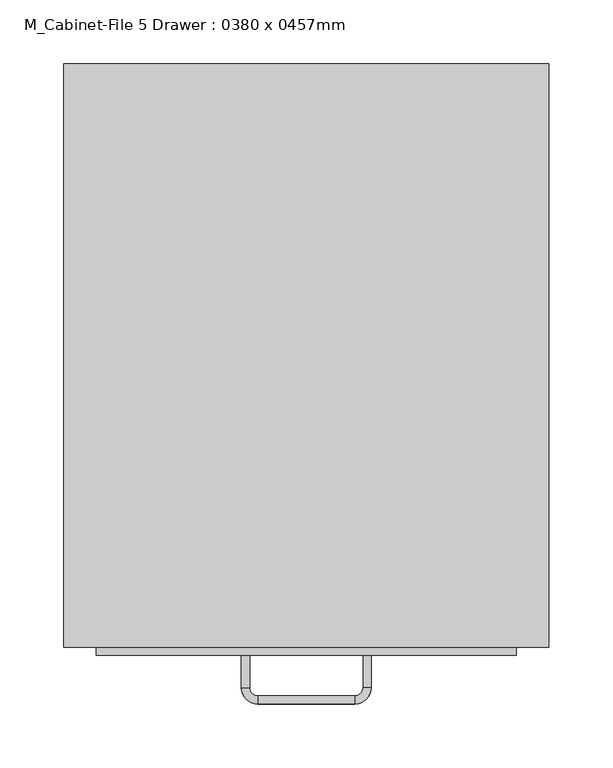
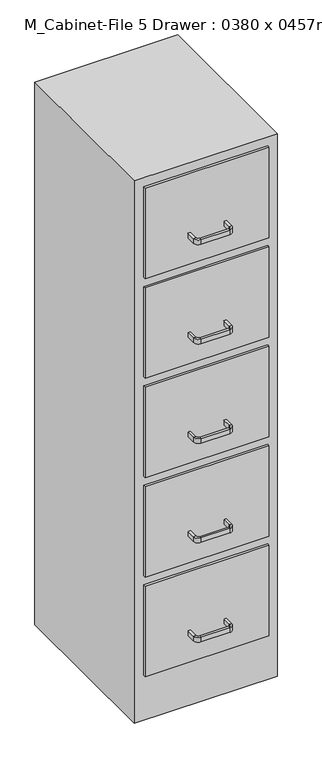
"""IFC4 building model written with IfcOpenShell, lengths in millimetres: furniture geometry, M_Cabinet-File 5 Drawer : 0380 x 0457mm."""

from ifc_helpers import new_model, si_unit, frame, origin, origin_with_axes, place, context, project, spatial, polyline, circle_curve, outline, extrude, source, transform, mapped, element, save
from ifc_brep_helpers import plane_surface, cylinder_surface, revolved_surface, advanced_brep


def m_cabinet_file_5_drawer_0380_x_0457mm_21dee09a(model_context):
    return source(origin(), model_context, "Body", "SolidModel", [
        extrude(outline(polyline([(36.703553, -376.9843001), (-292.496447, -376.9843001), (-292.496447, -370.6343001), (36.703553, -370.6343001), (36.703553, -376.9843001)])), frame((0.0, 0.0, 1244.6), z_axis=(0.0, 0.0, 1.0), x_axis=(1.0, 0.0, 0.0)), (0.0, 0.0, 1.0), 255.0),
        extrude(outline(polyline([(36.703553, -376.9843001), (-292.496447, -376.9843001), (-292.496447, -370.6343001), (36.703553, -370.6343001), (36.703553, -376.9843001)])), frame((0.0, 0.0, 965.2), z_axis=(0.0, 0.0, 1.0), x_axis=(1.0, 0.0, 0.0)), (0.0, 0.0, 1.0), 254.0),
        extrude(outline(polyline([(36.703553, -376.9843001), (-292.496447, -376.9843001), (-292.496447, -370.6343001), (36.703553, -370.6343001), (36.703553, -376.9843001)])), frame((0.0, 0.0, 685.8), z_axis=(0.0, 0.0, 1.0), x_axis=(1.0, 0.0, 0.0)), (0.0, 0.0, 1.0), 254.0),
        extrude(outline(polyline([(36.703553, -376.9843001), (-292.496447, -376.9843001), (-292.496447, -370.6343001), (36.703553, -370.6343001), (36.703553, -376.9843001)])), frame((0.0, 0.0, 406.4), z_axis=(0.0, 0.0, 1.0), x_axis=(1.0, 0.0, 0.0)), (0.0, 0.0, 1.0), 254.0),
        extrude(outline(polyline([(36.703553, -376.9843001), (-292.496447, -376.9843001), (-292.496447, -370.6343001), (36.703553, -370.6343001), (36.703553, -376.9843001)])), frame((0.0, 0.0, 127.0), z_axis=(0.0, 0.0, 1.0), x_axis=(1.0, 0.0, 0.0)), (0.0, 0.0, 1.0), 254.0),
        extrude(outline(polyline([(62.103553, 86.3656999), (62.103553, -370.6343001), (-317.896447, -370.6343001), (-317.896447, 86.3656999), (62.103553, 86.3656999)])), origin_with_axes(), (0.0, 0.0, 1.0), 1525.0),
        advanced_brep(
        [(-172.346447, -376.9843001, 203.2), (-178.696447, -376.9843001, 203.2), (-178.696447, -376.9843001, 215.9), (-172.346447, -376.9843001, 215.9), (-172.346447, -402.3843001, 203.2), (-178.696447, -402.3843001, 203.2), (-178.696447, -402.3843001, 215.9), (-172.346447, -402.3843001, 215.9), (-165.996447, -415.0843001, 203.2), (-165.996447, -408.7343001, 203.2), (-165.996447, -415.0843001, 215.9), (-165.996447, -408.7343001, 215.9), (-89.796447, -408.7343001, 203.2), (-89.796447, -415.0843001, 203.2), (-89.796447, -415.0843001, 215.9), (-89.796447, -408.7343001, 215.9), (-77.096447, -402.3843001, 203.2), (-83.446447, -402.3843001, 203.2), (-77.096447, -402.3843001, 215.9), (-83.446447, -402.3843001, 215.9), (-83.446447, -376.9843001, 203.2), (-83.446447, -376.9843001, 215.9), (-77.096447, -376.9843001, 215.9), (-77.096447, -376.9843001, 203.2)],
        [
            (0, 1),
            (1, 2),
            (2, 3),
            (3, 0),
            (0, 4),
            (4, 5),
            (5, 1),
            (5, 6),
            (6, 2),
            (6, 7),
            (7, 3),
            (7, 4),
            (8, 5, circle_curve(frame((-165.996447, -402.3843001, 203.2), z_axis=(0.0, 0.0, -1.0), x_axis=(-1.0, 0.0, 0.0)), 12.7)),
            (4, 9, circle_curve(frame((-165.996447, -402.3843001, 203.2), z_axis=(0.0, 0.0, 1.0), x_axis=(-1.0, 0.0, 0.0)), 6.35)),
            (9, 8),
            (10, 6, circle_curve(frame((-165.996447, -402.3843001, 215.9), z_axis=(0.0, 0.0, -1.0), x_axis=(-1.0, 0.0, 0.0)), 12.7)),
            (8, 10),
            (11, 7, circle_curve(frame((-165.996447, -402.3843001, 215.9), z_axis=(0.0, 0.0, -1.0), x_axis=(-1.0, 0.0, 0.0)), 6.35)),
            (10, 11),
            (11, 9),
            (9, 12),
            (12, 13),
            (13, 8),
            (13, 14),
            (14, 10),
            (14, 15),
            (15, 11),
            (15, 12),
            (16, 13, circle_curve(frame((-89.796447, -402.3843001, 203.2), z_axis=(0.0, 0.0, -1.0), x_axis=(0.0, -1.0, 0.0)), 12.7)),
            (12, 17, circle_curve(frame((-89.796447, -402.3843001, 203.2), z_axis=(0.0, 0.0, 1.0), x_axis=(0.0, -1.0, 0.0)), 6.35)),
            (17, 16),
            (18, 14, circle_curve(frame((-89.796447, -402.3843001, 215.9), z_axis=(0.0, 0.0, -1.0), x_axis=(0.0, -1.0, 0.0)), 12.7)),
            (16, 18),
            (19, 15, circle_curve(frame((-89.796447, -402.3843001, 215.9), z_axis=(0.0, 0.0, -1.0), x_axis=(0.0, -1.0, 0.0)), 6.35)),
            (18, 19),
            (19, 17),
            (20, 21),
            (21, 22),
            (22, 23),
            (23, 20),
            (17, 20),
            (23, 16),
            (22, 18),
            (21, 19),
        ],
        [
            plane_surface(frame((-1512.211566, -376.9843001, 0.0), z_axis=(0.0, 1.0, 0.0), x_axis=(0.0, 0.0, -1.0))),
            plane_surface(frame((-172.346447, -376.9843001, 203.2), z_axis=(0.0, 0.0, -1.0), x_axis=(0.0, -1.0, 0.0))),
            plane_surface(frame((-178.696447, -376.9843001, 203.2), z_axis=(-1.0, 0.0, 0.0), x_axis=(0.0, -1.0, 0.0))),
            plane_surface(frame((-178.696447, -376.9843001, 215.9), z_axis=(0.0, 0.0, 1.0), x_axis=(0.0, -1.0, 0.0))),
            plane_surface(frame((-172.346447, -376.9843001, 215.9), z_axis=(1.0, 0.0, 0.0), x_axis=(0.0, -1.0, 0.0))),
            plane_surface(frame((-165.996447, -402.3843001, 203.2), z_axis=(0.0, 0.0, -1.0), x_axis=(-1.0, 0.0, 0.0))),
            cylinder_surface(frame((-165.996447, -402.3843001, 0.0), z_axis=(0.0, 0.0, 1.0), x_axis=(-1.0, 0.0, 0.0)), 12.7),
            plane_surface(frame((-165.996447, -402.3843001, 215.9), z_axis=(0.0, 0.0, 1.0), x_axis=(-1.0, 0.0, 0.0))),
            revolved_surface(polyline([(-172.34644699999998, -402.3843001, 215.9), (-172.34644699999998, -402.3843001, 203.2)]), (-165.996447, -402.3843001, 0.0), (0.0, 0.0, 1.0)),
            plane_surface(frame((-165.996447, -408.7343001, 203.2), z_axis=(0.0, 0.0, -1.0), x_axis=(1.0, 0.0, 0.0))),
            plane_surface(frame((-165.996447, -415.0843001, 203.2), z_axis=(0.0, -1.0, 0.0), x_axis=(1.0, 0.0, 0.0))),
            plane_surface(frame((-165.996447, -415.0843001, 215.9), z_axis=(0.0, 0.0, 1.0), x_axis=(1.0, 0.0, 0.0))),
            plane_surface(frame((-165.996447, -408.7343001, 215.9), z_axis=(0.0, 1.0, 0.0), x_axis=(1.0, 0.0, 0.0))),
            plane_surface(frame((-89.796447, -402.3843001, 203.2), z_axis=(0.0, 0.0, -1.0), x_axis=(0.0, -1.0, 0.0))),
            cylinder_surface(frame((-89.796447, -402.3843001, 0.0), z_axis=(0.0, 0.0, 1.0), x_axis=(0.0, -1.0, 0.0)), 12.7),
            plane_surface(frame((-89.796447, -402.3843001, 215.9), z_axis=(0.0, 0.0, 1.0), x_axis=(0.0, -1.0, 0.0))),
            revolved_surface(polyline([(-89.796447, -408.73430010000004, 215.9), (-89.796447, -408.73430010000004, 203.2)]), (-89.796447, -402.3843001, 0.0), (0.0, 0.0, 1.0)),
            plane_surface(frame((-1410.611566, -376.9843001, 0.0), z_axis=(0.0, 1.0, 0.0), x_axis=(0.0, 0.0, 1.0))),
            plane_surface(frame((-83.446447, -402.3843001, 203.2), z_axis=(0.0, 0.0, -1.0), x_axis=(0.0, 1.0, 0.0))),
            plane_surface(frame((-77.096447, -402.3843001, 203.2), z_axis=(1.0, 0.0, 0.0), x_axis=(0.0, 1.0, 0.0))),
            plane_surface(frame((-77.096447, -402.3843001, 215.9), z_axis=(0.0, 0.0, 1.0), x_axis=(0.0, 1.0, 0.0))),
            plane_surface(frame((-83.446447, -402.3843001, 215.9), z_axis=(-1.0, 0.0, 0.0), x_axis=(0.0, 1.0, 0.0))),
        ],
        [
            (0, [[1, 2, 3, 4]]),
            (1, [[-1, 5, 6, 7]]),
            (2, [[-2, -7, 8, 9]]),
            (3, [[-3, -9, 10, 11]]),
            (4, [[-4, -11, 12, -5]]),
            (5, [[13, -6, 14, 15]]),
            (6, [[16, -8, -13, 17]]),
            (7, [[18, -10, -16, 19]]),
            (8, [[-14, -12, -18, 20]]),
            (9, [[-15, 21, 22, 23]]),
            (10, [[-17, -23, 24, 25]]),
            (11, [[-19, -25, 26, 27]]),
            (12, [[-20, -27, 28, -21]]),
            (13, [[29, -22, 30, 31]]),
            (14, [[32, -24, -29, 33]]),
            (15, [[34, -26, -32, 35]]),
            (16, [[-30, -28, -34, 36]]),
            (17, [[37, 38, 39, 40]]),
            (18, [[-31, 41, -40, 42]]),
            (19, [[-33, -42, -39, 43]]),
            (20, [[-35, -43, -38, 44]]),
            (21, [[-36, -44, -37, -41]]),
        ],
    ),
        advanced_brep(
        [(-172.346447, -376.9843001, 482.6), (-178.696447, -376.9843001, 482.6), (-178.696447, -376.9843001, 495.3), (-172.346447, -376.9843001, 495.3), (-172.346447, -402.3843001, 482.6), (-178.696447, -402.3843001, 482.6), (-178.696447, -402.3843001, 495.3), (-172.346447, -402.3843001, 495.3), (-165.996447, -415.0843001, 482.6), (-165.996447, -408.7343001, 482.6), (-165.996447, -415.0843001, 495.3), (-165.996447, -408.7343001, 495.3), (-89.796447, -408.7343001, 482.6), (-89.796447, -415.0843001, 482.6), (-89.796447, -415.0843001, 495.3), (-89.796447, -408.7343001, 495.3), (-77.096447, -402.3843001, 482.6), (-83.446447, -402.3843001, 482.6), (-77.096447, -402.3843001, 495.3), (-83.446447, -402.3843001, 495.3), (-83.446447, -376.9843001, 482.6), (-83.446447, -376.9843001, 495.3), (-77.096447, -376.9843001, 495.3), (-77.096447, -376.9843001, 482.6)],
        [
            (0, 1),
            (1, 2),
            (2, 3),
            (3, 0),
            (0, 4),
            (4, 5),
            (5, 1),
            (5, 6),
            (6, 2),
            (6, 7),
            (7, 3),
            (7, 4),
            (8, 5, circle_curve(frame((-165.996447, -402.3843001, 482.6), z_axis=(0.0, 0.0, -1.0), x_axis=(-1.0, 0.0, 0.0)), 12.7)),
            (4, 9, circle_curve(frame((-165.996447, -402.3843001, 482.6), z_axis=(0.0, 0.0, 1.0), x_axis=(-1.0, 0.0, 0.0)), 6.35)),
            (9, 8),
            (10, 6, circle_curve(frame((-165.996447, -402.3843001, 495.3), z_axis=(0.0, 0.0, -1.0), x_axis=(-1.0, 0.0, 0.0)), 12.7)),
            (8, 10),
            (11, 7, circle_curve(frame((-165.996447, -402.3843001, 495.3), z_axis=(0.0, 0.0, -1.0), x_axis=(-1.0, 0.0, 0.0)), 6.35)),
            (10, 11),
            (11, 9),
            (9, 12),
            (12, 13),
            (13, 8),
            (13, 14),
            (14, 10),
            (14, 15),
            (15, 11),
            (15, 12),
            (16, 13, circle_curve(frame((-89.796447, -402.3843001, 482.6), z_axis=(0.0, 0.0, -1.0), x_axis=(0.0, -1.0, 0.0)), 12.7)),
            (12, 17, circle_curve(frame((-89.796447, -402.3843001, 482.6), z_axis=(0.0, 0.0, 1.0), x_axis=(0.0, -1.0, 0.0)), 6.35)),
            (17, 16),
            (18, 14, circle_curve(frame((-89.796447, -402.3843001, 495.3), z_axis=(0.0, 0.0, -1.0), x_axis=(0.0, -1.0, 0.0)), 12.7)),
            (16, 18),
            (19, 15, circle_curve(frame((-89.796447, -402.3843001, 495.3), z_axis=(0.0, 0.0, -1.0), x_axis=(0.0, -1.0, 0.0)), 6.35)),
            (18, 19),
            (19, 17),
            (20, 21),
            (21, 22),
            (22, 23),
            (23, 20),
            (17, 20),
            (23, 16),
            (22, 18),
            (21, 19),
        ],
        [
            plane_surface(frame((-1512.211566, -376.9843001, 0.0), z_axis=(0.0, 1.0, 0.0), x_axis=(0.0, 0.0, -1.0))),
            plane_surface(frame((-172.346447, -376.9843001, 482.6), z_axis=(0.0, 0.0, -1.0), x_axis=(0.0, -1.0, 0.0))),
            plane_surface(frame((-178.696447, -376.9843001, 482.6), z_axis=(-1.0, 0.0, 0.0), x_axis=(0.0, -1.0, 0.0))),
            plane_surface(frame((-178.696447, -376.9843001, 495.3), z_axis=(0.0, 0.0, 1.0), x_axis=(0.0, -1.0, 0.0))),
            plane_surface(frame((-172.346447, -376.9843001, 495.3), z_axis=(1.0, 0.0, 0.0), x_axis=(0.0, -1.0, 0.0))),
            plane_surface(frame((-165.996447, -402.3843001, 482.6), z_axis=(0.0, 0.0, -1.0), x_axis=(-1.0, 0.0, 0.0))),
            cylinder_surface(frame((-165.996447, -402.3843001, 0.0), z_axis=(0.0, 0.0, 1.0), x_axis=(-1.0, 0.0, 0.0)), 12.7),
            plane_surface(frame((-165.996447, -402.3843001, 495.3), z_axis=(0.0, 0.0, 1.0), x_axis=(-1.0, 0.0, 0.0))),
            revolved_surface(polyline([(-172.34644699999998, -402.3843001, 495.3), (-172.34644699999998, -402.3843001, 482.6)]), (-165.996447, -402.3843001, 0.0), (0.0, 0.0, 1.0)),
            plane_surface(frame((-165.996447, -408.7343001, 482.6), z_axis=(0.0, 0.0, -1.0), x_axis=(1.0, 0.0, 0.0))),
            plane_surface(frame((-165.996447, -415.0843001, 482.6), z_axis=(0.0, -1.0, 0.0), x_axis=(1.0, 0.0, 0.0))),
            plane_surface(frame((-165.996447, -415.0843001, 495.3), z_axis=(0.0, 0.0, 1.0), x_axis=(1.0, 0.0, 0.0))),
            plane_surface(frame((-165.996447, -408.7343001, 495.3), z_axis=(0.0, 1.0, 0.0), x_axis=(1.0, 0.0, 0.0))),
            plane_surface(frame((-89.796447, -402.3843001, 482.6), z_axis=(0.0, 0.0, -1.0), x_axis=(0.0, -1.0, 0.0))),
            cylinder_surface(frame((-89.796447, -402.3843001, 0.0), z_axis=(0.0, 0.0, 1.0), x_axis=(0.0, -1.0, 0.0)), 12.7),
            plane_surface(frame((-89.796447, -402.3843001, 495.3), z_axis=(0.0, 0.0, 1.0), x_axis=(0.0, -1.0, 0.0))),
            revolved_surface(polyline([(-89.796447, -408.73430010000004, 495.3), (-89.796447, -408.73430010000004, 482.6)]), (-89.796447, -402.3843001, 0.0), (0.0, 0.0, 1.0)),
            plane_surface(frame((-1410.611566, -376.9843001, 0.0), z_axis=(0.0, 1.0, 0.0), x_axis=(0.0, 0.0, 1.0))),
            plane_surface(frame((-83.446447, -402.3843001, 482.6), z_axis=(0.0, 0.0, -1.0), x_axis=(0.0, 1.0, 0.0))),
            plane_surface(frame((-77.096447, -402.3843001, 482.6), z_axis=(1.0, 0.0, 0.0), x_axis=(0.0, 1.0, 0.0))),
            plane_surface(frame((-77.096447, -402.3843001, 495.3), z_axis=(0.0, 0.0, 1.0), x_axis=(0.0, 1.0, 0.0))),
            plane_surface(frame((-83.446447, -402.3843001, 495.3), z_axis=(-1.0, 0.0, 0.0), x_axis=(0.0, 1.0, 0.0))),
        ],
        [
            (0, [[1, 2, 3, 4]]),
            (1, [[-1, 5, 6, 7]]),
            (2, [[-2, -7, 8, 9]]),
            (3, [[-3, -9, 10, 11]]),
            (4, [[-4, -11, 12, -5]]),
            (5, [[13, -6, 14, 15]]),
            (6, [[16, -8, -13, 17]]),
            (7, [[18, -10, -16, 19]]),
            (8, [[-14, -12, -18, 20]]),
            (9, [[-15, 21, 22, 23]]),
            (10, [[-17, -23, 24, 25]]),
            (11, [[-19, -25, 26, 27]]),
            (12, [[-20, -27, 28, -21]]),
            (13, [[29, -22, 30, 31]]),
            (14, [[32, -24, -29, 33]]),
            (15, [[34, -26, -32, 35]]),
            (16, [[-30, -28, -34, 36]]),
            (17, [[37, 38, 39, 40]]),
            (18, [[-31, 41, -40, 42]]),
            (19, [[-33, -42, -39, 43]]),
            (20, [[-35, -43, -38, 44]]),
            (21, [[-36, -44, -37, -41]]),
        ],
    ),
        advanced_brep(
        [(-172.346447, -376.9843001, 762.0), (-178.696447, -376.9843001, 762.0), (-178.696447, -376.9843001, 774.7), (-172.346447, -376.9843001, 774.7), (-172.346447, -402.3843001, 762.0), (-178.696447, -402.3843001, 762.0), (-178.696447, -402.3843001, 774.7), (-172.346447, -402.3843001, 774.7), (-165.996447, -415.0843001, 762.0), (-165.996447, -408.7343001, 762.0), (-165.996447, -415.0843001, 774.7), (-165.996447, -408.7343001, 774.7), (-89.796447, -408.7343001, 762.0), (-89.796447, -415.0843001, 762.0), (-89.796447, -415.0843001, 774.7), (-89.796447, -408.7343001, 774.7), (-77.096447, -402.3843001, 762.0), (-83.446447, -402.3843001, 762.0), (-77.096447, -402.3843001, 774.7), (-83.446447, -402.3843001, 774.7), (-83.446447, -376.9843001, 762.0), (-83.446447, -376.9843001, 774.7), (-77.096447, -376.9843001, 774.7), (-77.096447, -376.9843001, 762.0)],
        [
            (0, 1),
            (1, 2),
            (2, 3),
            (3, 0),
            (0, 4),
            (4, 5),
            (5, 1),
            (5, 6),
            (6, 2),
            (6, 7),
            (7, 3),
            (7, 4),
            (8, 5, circle_curve(frame((-165.996447, -402.3843001, 762.0), z_axis=(0.0, 0.0, -1.0), x_axis=(-1.0, 0.0, 0.0)), 12.7)),
            (4, 9, circle_curve(frame((-165.996447, -402.3843001, 762.0), z_axis=(0.0, 0.0, 1.0), x_axis=(-1.0, 0.0, 0.0)), 6.35)),
            (9, 8),
            (10, 6, circle_curve(frame((-165.996447, -402.3843001, 774.7), z_axis=(0.0, 0.0, -1.0), x_axis=(-1.0, 0.0, 0.0)), 12.7)),
            (8, 10),
            (11, 7, circle_curve(frame((-165.996447, -402.3843001, 774.7), z_axis=(0.0, 0.0, -1.0), x_axis=(-1.0, 0.0, 0.0)), 6.35)),
            (10, 11),
            (11, 9),
            (9, 12),
            (12, 13),
            (13, 8),
            (13, 14),
            (14, 10),
            (14, 15),
            (15, 11),
            (15, 12),
            (16, 13, circle_curve(frame((-89.796447, -402.3843001, 762.0), z_axis=(0.0, 0.0, -1.0), x_axis=(0.0, -1.0, 0.0)), 12.7)),
            (12, 17, circle_curve(frame((-89.796447, -402.3843001, 762.0), z_axis=(0.0, 0.0, 1.0), x_axis=(0.0, -1.0, 0.0)), 6.35)),
            (17, 16),
            (18, 14, circle_curve(frame((-89.796447, -402.3843001, 774.7), z_axis=(0.0, 0.0, -1.0), x_axis=(0.0, -1.0, 0.0)), 12.7)),
            (16, 18),
            (19, 15, circle_curve(frame((-89.796447, -402.3843001, 774.7), z_axis=(0.0, 0.0, -1.0), x_axis=(0.0, -1.0, 0.0)), 6.35)),
            (18, 19),
            (19, 17),
            (20, 21),
            (21, 22),
            (22, 23),
            (23, 20),
            (17, 20),
            (23, 16),
            (22, 18),
            (21, 19),
        ],
        [
            plane_surface(frame((-1512.211566, -376.9843001, 0.0), z_axis=(0.0, 1.0, 0.0), x_axis=(0.0, 0.0, -1.0))),
            plane_surface(frame((-172.346447, -376.9843001, 762.0), z_axis=(0.0, 0.0, -1.0), x_axis=(0.0, -1.0, 0.0))),
            plane_surface(frame((-178.696447, -376.9843001, 762.0), z_axis=(-1.0, 0.0, 0.0), x_axis=(0.0, -1.0, 0.0))),
            plane_surface(frame((-178.696447, -376.9843001, 774.7), z_axis=(0.0, 0.0, 1.0), x_axis=(0.0, -1.0, 0.0))),
            plane_surface(frame((-172.346447, -376.9843001, 774.7), z_axis=(1.0, 0.0, 0.0), x_axis=(0.0, -1.0, 0.0))),
            plane_surface(frame((-165.996447, -402.3843001, 762.0), z_axis=(0.0, 0.0, -1.0), x_axis=(-1.0, 0.0, 0.0))),
            cylinder_surface(frame((-165.996447, -402.3843001, 0.0), z_axis=(0.0, 0.0, 1.0), x_axis=(-1.0, 0.0, 0.0)), 12.7),
            plane_surface(frame((-165.996447, -402.3843001, 774.7), z_axis=(0.0, 0.0, 1.0), x_axis=(-1.0, 0.0, 0.0))),
            revolved_surface(polyline([(-172.34644699999998, -402.3843001, 774.7), (-172.34644699999998, -402.3843001, 762.0)]), (-165.996447, -402.3843001, 0.0), (0.0, 0.0, 1.0)),
            plane_surface(frame((-165.996447, -408.7343001, 762.0), z_axis=(0.0, 0.0, -1.0), x_axis=(1.0, 0.0, 0.0))),
            plane_surface(frame((-165.996447, -415.0843001, 762.0), z_axis=(0.0, -1.0, 0.0), x_axis=(1.0, 0.0, 0.0))),
            plane_surface(frame((-165.996447, -415.0843001, 774.7), z_axis=(0.0, 0.0, 1.0), x_axis=(1.0, 0.0, 0.0))),
            plane_surface(frame((-165.996447, -408.7343001, 774.7), z_axis=(0.0, 1.0, 0.0), x_axis=(1.0, 0.0, 0.0))),
            plane_surface(frame((-89.796447, -402.3843001, 762.0), z_axis=(0.0, 0.0, -1.0), x_axis=(0.0, -1.0, 0.0))),
            cylinder_surface(frame((-89.796447, -402.3843001, 0.0), z_axis=(0.0, 0.0, 1.0), x_axis=(0.0, -1.0, 0.0)), 12.7),
            plane_surface(frame((-89.796447, -402.3843001, 774.7), z_axis=(0.0, 0.0, 1.0), x_axis=(0.0, -1.0, 0.0))),
            revolved_surface(polyline([(-89.796447, -408.73430010000004, 774.7), (-89.796447, -408.73430010000004, 762.0)]), (-89.796447, -402.3843001, 0.0), (0.0, 0.0, 1.0)),
            plane_surface(frame((-1410.611566, -376.9843001, 0.0), z_axis=(0.0, 1.0, 0.0), x_axis=(0.0, 0.0, 1.0))),
            plane_surface(frame((-83.446447, -402.3843001, 762.0), z_axis=(0.0, 0.0, -1.0), x_axis=(0.0, 1.0, 0.0))),
            plane_surface(frame((-77.096447, -402.3843001, 762.0), z_axis=(1.0, 0.0, 0.0), x_axis=(0.0, 1.0, 0.0))),
            plane_surface(frame((-77.096447, -402.3843001, 774.7), z_axis=(0.0, 0.0, 1.0), x_axis=(0.0, 1.0, 0.0))),
            plane_surface(frame((-83.446447, -402.3843001, 774.7), z_axis=(-1.0, 0.0, 0.0), x_axis=(0.0, 1.0, 0.0))),
        ],
        [
            (0, [[1, 2, 3, 4]]),
            (1, [[-1, 5, 6, 7]]),
            (2, [[-2, -7, 8, 9]]),
            (3, [[-3, -9, 10, 11]]),
            (4, [[-4, -11, 12, -5]]),
            (5, [[13, -6, 14, 15]]),
            (6, [[16, -8, -13, 17]]),
            (7, [[18, -10, -16, 19]]),
            (8, [[-14, -12, -18, 20]]),
            (9, [[-15, 21, 22, 23]]),
            (10, [[-17, -23, 24, 25]]),
            (11, [[-19, -25, 26, 27]]),
            (12, [[-20, -27, 28, -21]]),
            (13, [[29, -22, 30, 31]]),
            (14, [[32, -24, -29, 33]]),
            (15, [[34, -26, -32, 35]]),
            (16, [[-30, -28, -34, 36]]),
            (17, [[37, 38, 39, 40]]),
            (18, [[-31, 41, -40, 42]]),
            (19, [[-33, -42, -39, 43]]),
            (20, [[-35, -43, -38, 44]]),
            (21, [[-36, -44, -37, -41]]),
        ],
    ),
        advanced_brep(
        [(-172.346447, -376.9843001, 1041.4), (-178.696447, -376.9843001, 1041.4), (-178.696447, -376.9843001, 1054.1), (-172.346447, -376.9843001, 1054.1), (-172.346447, -402.3843001, 1041.4), (-178.696447, -402.3843001, 1041.4), (-178.696447, -402.3843001, 1054.1), (-172.346447, -402.3843001, 1054.1), (-165.996447, -415.0843001, 1041.4), (-165.996447, -408.7343001, 1041.4), (-165.996447, -415.0843001, 1054.1), (-165.996447, -408.7343001, 1054.1), (-89.796447, -408.7343001, 1041.4), (-89.796447, -415.0843001, 1041.4), (-89.796447, -415.0843001, 1054.1), (-89.796447, -408.7343001, 1054.1), (-77.096447, -402.3843001, 1041.4), (-83.446447, -402.3843001, 1041.4), (-77.096447, -402.3843001, 1054.1), (-83.446447, -402.3843001, 1054.1), (-83.446447, -376.9843001, 1041.4), (-83.446447, -376.9843001, 1054.1), (-77.096447, -376.9843001, 1054.1), (-77.096447, -376.9843001, 1041.4)],
        [
            (0, 1),
            (1, 2),
            (2, 3),
            (3, 0),
            (0, 4),
            (4, 5),
            (5, 1),
            (5, 6),
            (6, 2),
            (6, 7),
            (7, 3),
            (7, 4),
            (8, 5, circle_curve(frame((-165.996447, -402.3843001, 1041.4), z_axis=(0.0, 0.0, -1.0), x_axis=(-1.0, 0.0, 0.0)), 12.7)),
            (4, 9, circle_curve(frame((-165.996447, -402.3843001, 1041.4), z_axis=(0.0, 0.0, 1.0), x_axis=(-1.0, 0.0, 0.0)), 6.35)),
            (9, 8),
            (10, 6, circle_curve(frame((-165.996447, -402.3843001, 1054.1), z_axis=(0.0, 0.0, -1.0), x_axis=(-1.0, 0.0, 0.0)), 12.7)),
            (8, 10),
            (11, 7, circle_curve(frame((-165.996447, -402.3843001, 1054.1), z_axis=(0.0, 0.0, -1.0), x_axis=(-1.0, 0.0, 0.0)), 6.35)),
            (10, 11),
            (11, 9),
            (9, 12),
            (12, 13),
            (13, 8),
            (13, 14),
            (14, 10),
            (14, 15),
            (15, 11),
            (15, 12),
            (16, 13, circle_curve(frame((-89.796447, -402.3843001, 1041.4), z_axis=(0.0, 0.0, -1.0), x_axis=(0.0, -1.0, 0.0)), 12.7)),
            (12, 17, circle_curve(frame((-89.796447, -402.3843001, 1041.4), z_axis=(0.0, 0.0, 1.0), x_axis=(0.0, -1.0, 0.0)), 6.35)),
            (17, 16),
            (18, 14, circle_curve(frame((-89.796447, -402.3843001, 1054.1), z_axis=(0.0, 0.0, -1.0), x_axis=(0.0, -1.0, 0.0)), 12.7)),
            (16, 18),
            (19, 15, circle_curve(frame((-89.796447, -402.3843001, 1054.1), z_axis=(0.0, 0.0, -1.0), x_axis=(0.0, -1.0, 0.0)), 6.35)),
            (18, 19),
            (19, 17),
            (20, 21),
            (21, 22),
            (22, 23),
            (23, 20),
            (17, 20),
            (23, 16),
            (22, 18),
            (21, 19),
        ],
        [
            plane_surface(frame((-1512.211566, -376.9843001, 0.0), z_axis=(0.0, 1.0, 0.0), x_axis=(0.0, 0.0, -1.0))),
            plane_surface(frame((-172.346447, -376.9843001, 1041.4), z_axis=(0.0, 0.0, -1.0), x_axis=(0.0, -1.0, 0.0))),
            plane_surface(frame((-178.696447, -376.9843001, 1041.4), z_axis=(-1.0, 0.0, 0.0), x_axis=(0.0, -1.0, 0.0))),
            plane_surface(frame((-178.696447, -376.9843001, 1054.1), z_axis=(0.0, 0.0, 1.0), x_axis=(0.0, -1.0, 0.0))),
            plane_surface(frame((-172.346447, -376.9843001, 1054.1), z_axis=(1.0, 0.0, 0.0), x_axis=(0.0, -1.0, 0.0))),
            plane_surface(frame((-165.996447, -402.3843001, 1041.4), z_axis=(0.0, 0.0, -1.0), x_axis=(-1.0, 0.0, 0.0))),
            cylinder_surface(frame((-165.996447, -402.3843001, 0.0), z_axis=(0.0, 0.0, 1.0), x_axis=(-1.0, 0.0, 0.0)), 12.7),
            plane_surface(frame((-165.996447, -402.3843001, 1054.1), z_axis=(0.0, 0.0, 1.0), x_axis=(-1.0, 0.0, 0.0))),
            revolved_surface(polyline([(-172.34644699999998, -402.3843001, 1054.1), (-172.34644699999998, -402.3843001, 1041.4)]), (-165.996447, -402.3843001, 0.0), (0.0, 0.0, 1.0)),
            plane_surface(frame((-165.996447, -408.7343001, 1041.4), z_axis=(0.0, 0.0, -1.0), x_axis=(1.0, 0.0, 0.0))),
            plane_surface(frame((-165.996447, -415.0843001, 1041.4), z_axis=(0.0, -1.0, 0.0), x_axis=(1.0, 0.0, 0.0))),
            plane_surface(frame((-165.996447, -415.0843001, 1054.1), z_axis=(0.0, 0.0, 1.0), x_axis=(1.0, 0.0, 0.0))),
            plane_surface(frame((-165.996447, -408.7343001, 1054.1), z_axis=(0.0, 1.0, 0.0), x_axis=(1.0, 0.0, 0.0))),
            plane_surface(frame((-89.796447, -402.3843001, 1041.4), z_axis=(0.0, 0.0, -1.0), x_axis=(0.0, -1.0, 0.0))),
            cylinder_surface(frame((-89.796447, -402.3843001, 0.0), z_axis=(0.0, 0.0, 1.0), x_axis=(0.0, -1.0, 0.0)), 12.7),
            plane_surface(frame((-89.796447, -402.3843001, 1054.1), z_axis=(0.0, 0.0, 1.0), x_axis=(0.0, -1.0, 0.0))),
            revolved_surface(polyline([(-89.796447, -408.73430010000004, 1054.1), (-89.796447, -408.73430010000004, 1041.4)]), (-89.796447, -402.3843001, 0.0), (0.0, 0.0, 1.0)),
            plane_surface(frame((-1410.611566, -376.9843001, 0.0), z_axis=(0.0, 1.0, 0.0), x_axis=(0.0, 0.0, 1.0))),
            plane_surface(frame((-83.446447, -402.3843001, 1041.4), z_axis=(0.0, 0.0, -1.0), x_axis=(0.0, 1.0, 0.0))),
            plane_surface(frame((-77.096447, -402.3843001, 1041.4), z_axis=(1.0, 0.0, 0.0), x_axis=(0.0, 1.0, 0.0))),
            plane_surface(frame((-77.096447, -402.3843001, 1054.1), z_axis=(0.0, 0.0, 1.0), x_axis=(0.0, 1.0, 0.0))),
            plane_surface(frame((-83.446447, -402.3843001, 1054.1), z_axis=(-1.0, 0.0, 0.0), x_axis=(0.0, 1.0, 0.0))),
        ],
        [
            (0, [[1, 2, 3, 4]]),
            (1, [[-1, 5, 6, 7]]),
            (2, [[-2, -7, 8, 9]]),
            (3, [[-3, -9, 10, 11]]),
            (4, [[-4, -11, 12, -5]]),
            (5, [[13, -6, 14, 15]]),
            (6, [[16, -8, -13, 17]]),
            (7, [[18, -10, -16, 19]]),
            (8, [[-14, -12, -18, 20]]),
            (9, [[-15, 21, 22, 23]]),
            (10, [[-17, -23, 24, 25]]),
            (11, [[-19, -25, 26, 27]]),
            (12, [[-20, -27, 28, -21]]),
            (13, [[29, -22, 30, 31]]),
            (14, [[32, -24, -29, 33]]),
            (15, [[34, -26, -32, 35]]),
            (16, [[-30, -28, -34, 36]]),
            (17, [[37, 38, 39, 40]]),
            (18, [[-31, 41, -40, 42]]),
            (19, [[-33, -42, -39, 43]]),
            (20, [[-35, -43, -38, 44]]),
            (21, [[-36, -44, -37, -41]]),
        ],
    ),
        advanced_brep(
        [(-172.346447, -376.9843001, 1320.8), (-178.696447, -376.9843001, 1320.8), (-178.696447, -376.9843001, 1333.5), (-172.346447, -376.9843001, 1333.5), (-172.346447, -402.3843001, 1320.8), (-178.696447, -402.3843001, 1320.8), (-178.696447, -402.3843001, 1333.5), (-172.346447, -402.3843001, 1333.5), (-165.996447, -415.0843001, 1320.8), (-165.996447, -408.7343001, 1320.8), (-165.996447, -415.0843001, 1333.5), (-165.996447, -408.7343001, 1333.5), (-89.796447, -408.7343001, 1320.8), (-89.796447, -415.0843001, 1320.8), (-89.796447, -415.0843001, 1333.5), (-89.796447, -408.7343001, 1333.5), (-77.096447, -402.3843001, 1320.8), (-83.446447, -402.3843001, 1320.8), (-77.096447, -402.3843001, 1333.5), (-83.446447, -402.3843001, 1333.5), (-83.446447, -376.9843001, 1320.8), (-83.446447, -376.9843001, 1333.5), (-77.096447, -376.9843001, 1333.5), (-77.096447, -376.9843001, 1320.8)],
        [
            (0, 1),
            (1, 2),
            (2, 3),
            (3, 0),
            (0, 4),
            (4, 5),
            (5, 1),
            (5, 6),
            (6, 2),
            (6, 7),
            (7, 3),
            (7, 4),
            (8, 5, circle_curve(frame((-165.996447, -402.3843001, 1320.8), z_axis=(0.0, 0.0, -1.0), x_axis=(-1.0, 0.0, 0.0)), 12.7)),
            (4, 9, circle_curve(frame((-165.996447, -402.3843001, 1320.8), z_axis=(0.0, 0.0, 1.0), x_axis=(-1.0, 0.0, 0.0)), 6.35)),
            (9, 8),
            (10, 6, circle_curve(frame((-165.996447, -402.3843001, 1333.5), z_axis=(0.0, 0.0, -1.0), x_axis=(-1.0, 0.0, 0.0)), 12.7)),
            (8, 10),
            (11, 7, circle_curve(frame((-165.996447, -402.3843001, 1333.5), z_axis=(0.0, 0.0, -1.0), x_axis=(-1.0, 0.0, 0.0)), 6.35)),
            (10, 11),
            (11, 9),
            (9, 12),
            (12, 13),
            (13, 8),
            (13, 14),
            (14, 10),
            (14, 15),
            (15, 11),
            (15, 12),
            (16, 13, circle_curve(frame((-89.796447, -402.3843001, 1320.8), z_axis=(0.0, 0.0, -1.0), x_axis=(0.0, -1.0, 0.0)), 12.7)),
            (12, 17, circle_curve(frame((-89.796447, -402.3843001, 1320.8), z_axis=(0.0, 0.0, 1.0), x_axis=(0.0, -1.0, 0.0)), 6.35)),
            (17, 16),
            (18, 14, circle_curve(frame((-89.796447, -402.3843001, 1333.5), z_axis=(0.0, 0.0, -1.0), x_axis=(0.0, -1.0, 0.0)), 12.7)),
            (16, 18),
            (19, 15, circle_curve(frame((-89.796447, -402.3843001, 1333.5), z_axis=(0.0, 0.0, -1.0), x_axis=(0.0, -1.0, 0.0)), 6.35)),
            (18, 19),
            (19, 17),
            (20, 21),
            (21, 22),
            (22, 23),
            (23, 20),
            (17, 20),
            (23, 16),
            (22, 18),
            (21, 19),
        ],
        [
            plane_surface(frame((-1512.211566, -376.9843001, 0.0), z_axis=(0.0, 1.0, 0.0), x_axis=(0.0, 0.0, -1.0))),
            plane_surface(frame((-172.346447, -376.9843001, 1320.8), z_axis=(0.0, 0.0, -1.0), x_axis=(0.0, -1.0, 0.0))),
            plane_surface(frame((-178.696447, -376.9843001, 1320.8), z_axis=(-1.0, 0.0, 0.0), x_axis=(0.0, -1.0, 0.0))),
            plane_surface(frame((-178.696447, -376.9843001, 1333.5), z_axis=(0.0, 0.0, 1.0), x_axis=(0.0, -1.0, 0.0))),
            plane_surface(frame((-172.346447, -376.9843001, 1333.5), z_axis=(1.0, 0.0, 0.0), x_axis=(0.0, -1.0, 0.0))),
            plane_surface(frame((-165.996447, -402.3843001, 1320.8), z_axis=(0.0, 0.0, -1.0), x_axis=(-1.0, 0.0, 0.0))),
            cylinder_surface(frame((-165.996447, -402.3843001, 0.0), z_axis=(0.0, 0.0, 1.0), x_axis=(-1.0, 0.0, 0.0)), 12.7),
            plane_surface(frame((-165.996447, -402.3843001, 1333.5), z_axis=(0.0, 0.0, 1.0), x_axis=(-1.0, 0.0, 0.0))),
            revolved_surface(polyline([(-172.34644699999998, -402.3843001, 1333.5), (-172.34644699999998, -402.3843001, 1320.8)]), (-165.996447, -402.3843001, 0.0), (0.0, 0.0, 1.0)),
            plane_surface(frame((-165.996447, -408.7343001, 1320.8), z_axis=(0.0, 0.0, -1.0), x_axis=(1.0, 0.0, 0.0))),
            plane_surface(frame((-165.996447, -415.0843001, 1320.8), z_axis=(0.0, -1.0, 0.0), x_axis=(1.0, 0.0, 0.0))),
            plane_surface(frame((-165.996447, -415.0843001, 1333.5), z_axis=(0.0, 0.0, 1.0), x_axis=(1.0, 0.0, 0.0))),
            plane_surface(frame((-165.996447, -408.7343001, 1333.5), z_axis=(0.0, 1.0, 0.0), x_axis=(1.0, 0.0, 0.0))),
            plane_surface(frame((-89.796447, -402.3843001, 1320.8), z_axis=(0.0, 0.0, -1.0), x_axis=(0.0, -1.0, 0.0))),
            cylinder_surface(frame((-89.796447, -402.3843001, 0.0), z_axis=(0.0, 0.0, 1.0), x_axis=(0.0, -1.0, 0.0)), 12.7),
            plane_surface(frame((-89.796447, -402.3843001, 1333.5), z_axis=(0.0, 0.0, 1.0), x_axis=(0.0, -1.0, 0.0))),
            revolved_surface(polyline([(-89.796447, -408.73430010000004, 1333.5), (-89.796447, -408.73430010000004, 1320.8)]), (-89.796447, -402.3843001, 0.0), (0.0, 0.0, 1.0)),
            plane_surface(frame((-1410.611566, -376.9843001, 0.0), z_axis=(0.0, 1.0, 0.0), x_axis=(0.0, 0.0, 1.0))),
            plane_surface(frame((-83.446447, -402.3843001, 1320.8), z_axis=(0.0, 0.0, -1.0), x_axis=(0.0, 1.0, 0.0))),
            plane_surface(frame((-77.096447, -402.3843001, 1320.8), z_axis=(1.0, 0.0, 0.0), x_axis=(0.0, 1.0, 0.0))),
            plane_surface(frame((-77.096447, -402.3843001, 1333.5), z_axis=(0.0, 0.0, 1.0), x_axis=(0.0, 1.0, 0.0))),
            plane_surface(frame((-83.446447, -402.3843001, 1333.5), z_axis=(-1.0, 0.0, 0.0), x_axis=(0.0, 1.0, 0.0))),
        ],
        [
            (0, [[1, 2, 3, 4]]),
            (1, [[-1, 5, 6, 7]]),
            (2, [[-2, -7, 8, 9]]),
            (3, [[-3, -9, 10, 11]]),
            (4, [[-4, -11, 12, -5]]),
            (5, [[13, -6, 14, 15]]),
            (6, [[16, -8, -13, 17]]),
            (7, [[18, -10, -16, 19]]),
            (8, [[-14, -12, -18, 20]]),
            (9, [[-15, 21, 22, 23]]),
            (10, [[-17, -23, 24, 25]]),
            (11, [[-19, -25, 26, 27]]),
            (12, [[-20, -27, 28, -21]]),
            (13, [[29, -22, 30, 31]]),
            (14, [[32, -24, -29, 33]]),
            (15, [[34, -26, -32, 35]]),
            (16, [[-30, -28, -34, 36]]),
            (17, [[37, 38, 39, 40]]),
            (18, [[-31, 41, -40, 42]]),
            (19, [[-33, -42, -39, 43]]),
            (20, [[-35, -43, -38, 44]]),
            (21, [[-36, -44, -37, -41]]),
        ],
    ),
    ])


if __name__ == "__main__":
    model = new_model("IFC4")
    model_context = context("Model", 3, world=origin())
    ifc_project = project(units=[si_unit("LENGTHUNIT", "METRE", prefix="MILLI")], contexts=[model_context])
    site = spatial("IfcSite", under=ifc_project)
    building = spatial("IfcBuilding", under=site)
    placement = place(None, origin())
    m_cabinet_file_5_drawer_0380_x_0457mm_shape = m_cabinet_file_5_drawer_0380_x_0457mm_21dee09a(model_context)
    element("IfcFurniture", 1, ObjectType="M_Cabinet-File 5 Drawer : 0380 x 0457mm", at=placement, inside=building, context=model_context, shape_type="MappedRepresentation", body=[
        mapped(m_cabinet_file_5_drawer_0380_x_0457mm_shape, transform((0.0, 0.0, 0.0), x_axis=(1.0, 0.0, 0.0), y_axis=(0.0, 1.0, 0.0), z_axis=(0.0, 0.0, 1.0))),
    ])
    save(model, "model.ifc")

# Revit data of these elements
# Type "M_Cabinet-File 5 Drawer : 0380 x 0457mm"
#   Depth = 1.499344 ft
#   Height = 5.003281 ft
#   Width = 1.246719 ft
#   Cabinet Material = Steel, Paint Finish, Ivory, Glossy
#   Handle Material = Steel, Chrome Plated
#   Default Elevation = 0
# Element 1 (IfcFurniture, "M_Cabinet-File 5 Drawer : 0380 x 0457mm")
#   Materials on its faces: "Steel, Chrome Plated", "Steel, Paint Finish, Ivory, Glossy"
# Materials
#   "Steel, Paint Finish, Ivory, Glossy": class "Metal", colour RGB 247 247 239, transparency 0, Description = "Steel, paint finish, ivory, glossy", Cost = 0
#   "Steel, Chrome Plated": class "Metal", colour RGB 17 17 17, transparency 0, Description = "Chromiuim plated steel", Cost = 0
